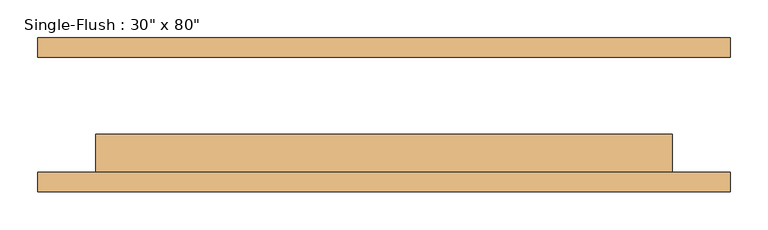
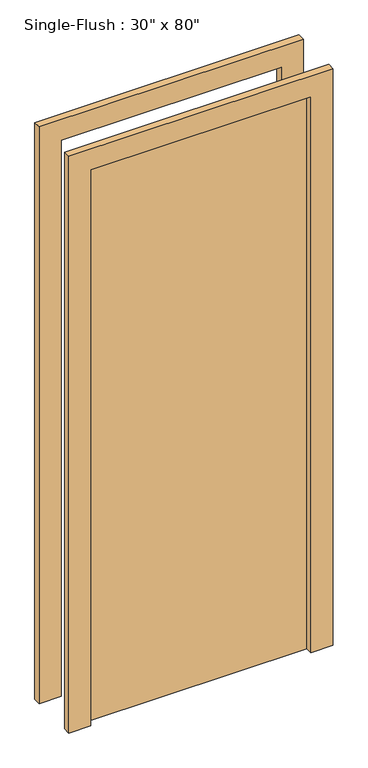
"""IFC4 building model written with IfcOpenShell, lengths in millimetres: door geometry."""

from ifc_helpers import new_model, si_unit, frame, origin, origin_with_axes, place, context, project, spatial, polyline, outline, extrude, source, transform, mapped, element, save


def door_255cab33(model_context):
    return source(origin(), model_context, "Body", "SweptSolid", [
        extrude(outline(polyline([(2108.2, -457.2), (0.0, -457.2), (0.0, -381.0), (2032.0, -381.0), (2032.0, 381.0), (0.0, 381.0), (0.0, 457.2), (2108.2, 457.2), (2108.2, -457.2)])), frame((0.0, -101.6, 0.0), z_axis=(0.0, 1.0, 0.0), x_axis=(0.0, 0.0, 1.0)), (0.0, 0.0, 1.0), 25.4),
        extrude(outline(polyline([(2108.2, 457.2), (2108.2, -457.2), (0.0, -457.2), (0.0, -381.0), (2032.0, -381.0), (2032.0, 381.0), (0.0, 381.0), (0.0, 457.2), (2108.2, 457.2)])), frame((0.0, 76.2, 0.0), z_axis=(0.0, 1.0, 0.0), x_axis=(0.0, 0.0, 1.0)), (0.0, 0.0, 1.0), 25.4),
        extrude(outline(polyline([(381.0, -25.4), (381.0, -76.2), (-381.0, -76.2), (-381.0, -25.4), (381.0, -25.4)])), origin_with_axes(), (0.0, 0.0, 1.0), 2032.0),
    ])


if __name__ == "__main__":
    model = new_model("IFC4")
    model_context = context("Model", 3, world=origin())
    ifc_project = project(units=[si_unit("LENGTHUNIT", "METRE", prefix="MILLI")], contexts=[model_context])
    site = spatial("IfcSite", under=ifc_project)
    building = spatial("IfcBuilding", under=site)
    placement = place(None, origin())
    door_shape = door_255cab33(model_context)
    element("IfcDoor", 1, ObjectType="Single-Flush : 30\" x 80\"", at=placement, inside=building, context=model_context, shape_type="MappedRepresentation", body=[
        mapped(door_shape, transform((0.0, 0.0, 0.0), x_axis=(1.0, 0.0, 0.0), y_axis=(0.0, 1.0, 0.0), z_axis=(0.0, 0.0, 1.0))),
    ])
    save(model, "model.ifc")

# Revit data of these elements
# Type "Single-Flush : 30\" x 80\""
#   Type Mark = "5"
#   Construction Type Id = "MDOOR"
#   Assembly Code = "C1020"
#   Analytic Construction = "Metal"
#   Thickness = 0' - 2"
#   Heat Transfer Coefficient (U) = 0.651978 BTU/(h·ft²·°F)
#   Height = 6' - 8"
#   Trim Projection Ext = 0' - 1"
#   Trim Projection Int = 0' - 1"
#   Trim Width = 0' - 3"
#   Width = 2' - 6"
#   Define Thermal Properties by = 1
#   Door Material = Door - Panel
#   Frame Material = Door - Frame
#   Visual Light Transmittance = 0
#   Solar Heat Gain Coefficient = 0
#   Function = (empty or 0)
#   Wall Closure = (empty or 0)
# Element 1 (IfcDoor, "Single-Flush : 30\" x 80\"")
#   Materials on its faces: "Door - Frame", "Door - Panel"
# Materials
#   "Door - Panel": class "Wood", colour RGB 210 159 95, transparency 0
#   "Door - Frame": colour RGB 118 70 51, transparency 0
